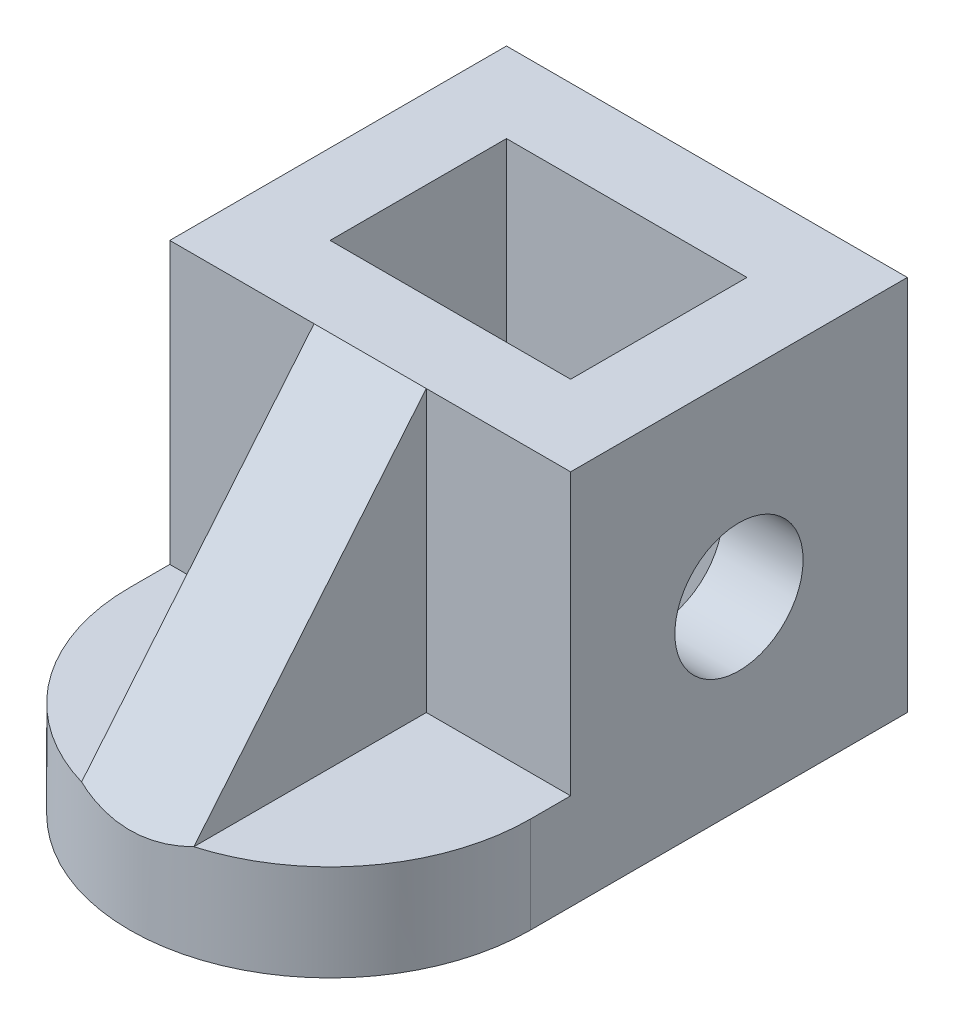
ISO-10303-21;
HEADER;
FILE_DESCRIPTION(('STEP AP214'),'2;1');
FILE_NAME('part.step','',(''),(''),'','','');
FILE_SCHEMA(('AUTOMOTIVE_DESIGN { 1 0 10303 214 1 1 1 1 }'));
ENDSEC;
DATA;
#1=APPLICATION_CONTEXT('core data for automotive mechanical design processes');
#2=APPLICATION_PROTOCOL_DEFINITION('international standard','automotive_design',2000,#1);
#3=PRODUCT_CONTEXT('',#1,'mechanical');
#4=PRODUCT('Part','Part','',(#3));
#5=PRODUCT_RELATED_PRODUCT_CATEGORY('part','',(#4));
#6=PRODUCT_DEFINITION_FORMATION('','',#4);
#7=PRODUCT_DEFINITION_CONTEXT('part definition',#1,'design');
#8=PRODUCT_DEFINITION('design','',#6,#7);
#9=PRODUCT_DEFINITION_SHAPE('','',#8);
#10=(LENGTH_UNIT() NAMED_UNIT(*) SI_UNIT(.MILLI.,.METRE.));
#11=(NAMED_UNIT(*) PLANE_ANGLE_UNIT() SI_UNIT($,.RADIAN.));
#12=(NAMED_UNIT(*) SI_UNIT($,.STERADIAN.) SOLID_ANGLE_UNIT());
#13=UNCERTAINTY_MEASURE_WITH_UNIT(LENGTH_MEASURE(1.E-05),#10,'distance_accuracy_value','');
#14=(GEOMETRIC_REPRESENTATION_CONTEXT(3) GLOBAL_UNCERTAINTY_ASSIGNED_CONTEXT((#13)) GLOBAL_UNIT_ASSIGNED_CONTEXT((#10,
#11,#12)) REPRESENTATION_CONTEXT('',''));
#15=CARTESIAN_POINT('',(0.,0.,0.));
#16=DIRECTION('',(0.,0.,1.));
#17=DIRECTION('',(1.,0.,0.));
#18=AXIS2_PLACEMENT_3D('',#15,#16,#17);
#19=CARTESIAN_POINT('',(-7.,23.5,15.));
#20=DIRECTION('',(1.,0.,0.));
#21=DIRECTION('',(0.,0.,-1.));
#22=AXIS2_PLACEMENT_3D('',#19,#20,#21);
#23=PLANE('',#22);
#24=DIRECTION('',(0.,-0.770021560905562,0.638017864750323));
#25=VECTOR('',#24,1.);
#26=CARTESIAN_POINT('',(-7.,12.,50.));
#27=LINE('',#26,#25);
#28=CARTESIAN_POINT('',(-7.,47.,21.));
#29=VERTEX_POINT('',#28);
#30=CARTESIAN_POINT('',(-7.,12.,50.));
#31=VERTEX_POINT('',#30);
#32=EDGE_CURVE('E146',#29,#31,#27,.T.);
#33=ORIENTED_EDGE('',*,*,#32,.F.);
#34=DIRECTION('',(0.,-1.,0.));
#35=VECTOR('',#34,1.);
#36=CARTESIAN_POINT('',(-7.,47.,21.));
#37=LINE('',#36,#35);
#38=CARTESIAN_POINT('',(-7.,12.,21.));
#39=VERTEX_POINT('',#38);
#40=EDGE_CURVE('E161',#29,#39,#37,.T.);
#41=ORIENTED_EDGE('',*,*,#40,.T.);
#42=DIRECTION('',(0.,0.,-1.));
#43=VECTOR('',#42,1.);
#44=CARTESIAN_POINT('',(-7.,12.,15.));
#45=LINE('',#44,#43);
#46=EDGE_CURVE('E56',#39,#31,#45,.F.);
#47=ORIENTED_EDGE('',*,*,#46,.T.);
#48=EDGE_LOOP('',(#33,#41,#47));
#49=FACE_BOUND('',#48,.T.);
#50=ADVANCED_FACE('F43',(#49),#23,.F.);
#51=CARTESIAN_POINT('',(7.,23.5,15.));
#52=DIRECTION('',(1.,0.,0.));
#53=DIRECTION('',(0.,0.,-1.));
#54=AXIS2_PLACEMENT_3D('',#51,#52,#53);
#55=PLANE('',#54);
#56=DIRECTION('',(0.,0.770021560905562,-0.638017864750323));
#57=VECTOR('',#56,1.);
#58=CARTESIAN_POINT('',(7.,12.,50.));
#59=LINE('',#58,#57);
#60=CARTESIAN_POINT('',(7.,12.,50.));
#61=VERTEX_POINT('',#60);
#62=CARTESIAN_POINT('',(7.,47.,21.));
#63=VERTEX_POINT('',#62);
#64=EDGE_CURVE('E158',#61,#63,#59,.T.);
#65=ORIENTED_EDGE('',*,*,#64,.F.);
#66=DIRECTION('',(0.,0.,-1.));
#67=VECTOR('',#66,1.);
#68=CARTESIAN_POINT('',(7.,12.,15.));
#69=LINE('',#68,#67);
#70=CARTESIAN_POINT('',(7.,12.,21.));
#71=VERTEX_POINT('',#70);
#72=EDGE_CURVE('E165',#71,#61,#69,.F.);
#73=ORIENTED_EDGE('',*,*,#72,.F.);
#74=DIRECTION('',(0.,-1.,0.));
#75=VECTOR('',#74,1.);
#76=CARTESIAN_POINT('',(7.,47.,21.));
#77=LINE('',#76,#75);
#78=EDGE_CURVE('E70',#63,#71,#77,.T.);
#79=ORIENTED_EDGE('',*,*,#78,.F.);
#80=EDGE_LOOP('',(#65,#73,#79));
#81=FACE_BOUND('',#80,.T.);
#82=ADVANCED_FACE('F279',(#81),#55,.T.);
#83=CARTESIAN_POINT('',(25.,47.,21.));
#84=DIRECTION('',(0.,0.,-1.));
#85=DIRECTION('',(-1.,0.,0.));
#86=AXIS2_PLACEMENT_3D('',#83,#84,#85);
#87=PLANE('',#86);
#88=ORIENTED_EDGE('',*,*,#40,.F.);
#89=DIRECTION('',(-1.,0.,0.));
#90=VECTOR('',#89,1.);
#91=CARTESIAN_POINT('',(25.,47.,21.));
#92=LINE('',#91,#90);
#93=CARTESIAN_POINT('',(-25.,47.,21.));
#94=VERTEX_POINT('',#93);
#95=EDGE_CURVE('E239',#29,#94,#92,.T.);
#96=ORIENTED_EDGE('',*,*,#95,.T.);
#97=DIRECTION('',(0.,-1.,0.));
#98=VECTOR('',#97,1.);
#99=CARTESIAN_POINT('',(-25.,47.,21.));
#100=LINE('',#99,#98);
#101=CARTESIAN_POINT('',(-25.,12.,21.));
#102=VERTEX_POINT('',#101);
#103=EDGE_CURVE('E234',#94,#102,#100,.T.);
#104=ORIENTED_EDGE('',*,*,#103,.T.);
#105=DIRECTION('',(-1.,0.,0.));
#106=VECTOR('',#105,1.);
#107=CARTESIAN_POINT('',(25.,12.,21.));
#108=LINE('',#107,#106);
#109=EDGE_CURVE('E228',#39,#102,#108,.T.);
#110=ORIENTED_EDGE('',*,*,#109,.F.);
#111=EDGE_LOOP('',(#88,#96,#104,#110));
#112=FACE_BOUND('',#111,.T.);
#113=ADVANCED_FACE('F288',(#112),#87,.F.);
#114=CARTESIAN_POINT('',(25.,12.,21.));
#115=DIRECTION('',(0.,-1.,0.));
#116=DIRECTION('',(0.,0.,-1.));
#117=AXIS2_PLACEMENT_3D('',#114,#115,#116);
#118=PLANE('',#117);
#119=ORIENTED_EDGE('',*,*,#46,.F.);
#120=ORIENTED_EDGE('',*,*,#109,.T.);
#121=DIRECTION('',(0.,0.,1.));
#122=VECTOR('',#121,1.);
#123=CARTESIAN_POINT('',(-25.,12.,21.));
#124=LINE('',#123,#122);
#125=CARTESIAN_POINT('',(-25.,12.,26.));
#126=VERTEX_POINT('',#125);
#127=EDGE_CURVE('E163',#102,#126,#124,.T.);
#128=ORIENTED_EDGE('',*,*,#127,.T.);
#129=CARTESIAN_POINT('',(0.,12.,26.));
#130=DIRECTION('',(0.,-1.,0.));
#131=DIRECTION('',(0.,0.,-1.));
#132=AXIS2_PLACEMENT_3D('',#129,#130,#131);
#133=CIRCLE('',#132,25.);
#134=EDGE_CURVE('E141',#126,#31,#133,.F.);
#135=ORIENTED_EDGE('',*,*,#134,.T.);
#136=EDGE_LOOP('',(#119,#120,#128,#135));
#137=FACE_BOUND('',#136,.T.);
#138=ADVANCED_FACE('F159',(#137),#118,.F.);
#139=CARTESIAN_POINT('',(25.,23.,0.));
#140=DIRECTION('',(-1.,0.,0.));
#141=DIRECTION('',(0.,0.,1.));
#142=AXIS2_PLACEMENT_3D('',#139,#140,#141);
#143=CYLINDRICAL_SURFACE('',#142,8.);
#144=CARTESIAN_POINT('',(15.,23.,0.));
#145=DIRECTION('',(1.,0.,0.));
#146=DIRECTION('',(0.,0.,-1.));
#147=AXIS2_PLACEMENT_3D('',#144,#145,#146);
#148=CIRCLE('',#147,8.);
#149=CARTESIAN_POINT('',(15.,23.,-8.));
#150=VERTEX_POINT('',#149);
#151=EDGE_CURVE('E179',#150,#150,#148,.F.);
#152=ORIENTED_EDGE('',*,*,#151,.T.);
#153=EDGE_LOOP('',(#152));
#154=FACE_BOUND('',#153,.T.);
#155=CARTESIAN_POINT('',(25.,23.,0.));
#156=DIRECTION('',(1.,0.,0.));
#157=DIRECTION('',(0.,0.,-1.));
#158=AXIS2_PLACEMENT_3D('',#155,#156,#157);
#159=CIRCLE('',#158,8.);
#160=CARTESIAN_POINT('',(25.,23.,-8.));
#161=VERTEX_POINT('',#160);
#162=EDGE_CURVE('E209',#161,#161,#159,.T.);
#163=ORIENTED_EDGE('',*,*,#162,.T.);
#164=EDGE_LOOP('',(#163));
#165=FACE_BOUND('',#164,.T.);
#166=ADVANCED_FACE('F321',(#154,#165),#143,.F.);
#167=CARTESIAN_POINT('',(0.,12.,26.));
#168=DIRECTION('',(0.,-1.,0.));
#169=DIRECTION('',(0.,0.,-1.));
#170=AXIS2_PLACEMENT_3D('',#167,#168,#169);
#171=CYLINDRICAL_SURFACE('',#170,25.);
#172=DIRECTION('',(0.,1.,0.));
#173=VECTOR('',#172,1.);
#174=CARTESIAN_POINT('',(25.,12.,26.));
#175=LINE('',#174,#173);
#176=CARTESIAN_POINT('',(25.,12.,26.));
#177=VERTEX_POINT('',#176);
#178=CARTESIAN_POINT('',(25.,0.,26.));
#179=VERTEX_POINT('',#178);
#180=EDGE_CURVE('E247',#177,#179,#175,.F.);
#181=ORIENTED_EDGE('',*,*,#180,.F.);
#182=EDGE_CURVE('E143',#61,#177,#133,.F.);
#183=ORIENTED_EDGE('',*,*,#182,.F.);
#184=CARTESIAN_POINT('',(0.,40.9655172413793,26.));
#185=DIRECTION('',(0.,-0.638017864750323,-0.770021560905562));
#186=DIRECTION('',(0.,-0.770021560905562,0.638017864750323));
#187=AXIS2_PLACEMENT_3D('',#184,#185,#186);
#188=ELLIPSE('',#187,39.1838557840121,25.);
#189=EDGE_CURVE('E11',#31,#61,#188,.F.);
#190=ORIENTED_EDGE('',*,*,#189,.F.);
#191=ORIENTED_EDGE('',*,*,#134,.F.);
#192=DIRECTION('',(0.,-1.,0.));
#193=VECTOR('',#192,1.);
#194=CARTESIAN_POINT('',(-25.,0.,26.));
#195=LINE('',#194,#193);
#196=CARTESIAN_POINT('',(-25.,0.,26.));
#197=VERTEX_POINT('',#196);
#198=EDGE_CURVE('E252',#197,#126,#195,.F.);
#199=ORIENTED_EDGE('',*,*,#198,.F.);
#200=CARTESIAN_POINT('',(0.,0.,26.));
#201=DIRECTION('',(0.,1.,0.));
#202=DIRECTION('',(0.,0.,1.));
#203=AXIS2_PLACEMENT_3D('',#200,#201,#202);
#204=CIRCLE('',#203,25.);
#205=EDGE_CURVE('E55',#179,#197,#204,.F.);
#206=ORIENTED_EDGE('',*,*,#205,.F.);
#207=EDGE_LOOP('',(#181,#183,#190,#191,#199,#206));
#208=FACE_BOUND('',#207,.T.);
#209=ADVANCED_FACE('F46',(#208),#171,.T.);
#210=CARTESIAN_POINT('',(25.,0.,0.));
#211=DIRECTION('',(1.,0.,0.));
#212=DIRECTION('',(0.,0.,-1.));
#213=AXIS2_PLACEMENT_3D('',#210,#211,#212);
#214=PLANE('',#213);
#215=DIRECTION('',(0.,0.,1.));
#216=VECTOR('',#215,1.);
#217=CARTESIAN_POINT('',(25.,12.,21.));
#218=LINE('',#217,#216);
#219=CARTESIAN_POINT('',(25.,12.,21.));
#220=VERTEX_POINT('',#219);
#221=EDGE_CURVE('E221',#220,#177,#218,.T.);
#222=ORIENTED_EDGE('',*,*,#221,.T.);
#223=ORIENTED_EDGE('',*,*,#180,.T.);
#224=DIRECTION('',(0.,0.,-1.));
#225=VECTOR('',#224,1.);
#226=CARTESIAN_POINT('',(25.,0.,51.));
#227=LINE('',#226,#225);
#228=CARTESIAN_POINT('',(25.,0.,-21.));
#229=VERTEX_POINT('',#228);
#230=EDGE_CURVE('E213',#179,#229,#227,.T.);
#231=ORIENTED_EDGE('',*,*,#230,.T.);
#232=DIRECTION('',(0.,1.,0.));
#233=VECTOR('',#232,1.);
#234=CARTESIAN_POINT('',(25.,0.,-21.));
#235=LINE('',#234,#233);
#236=CARTESIAN_POINT('',(25.,47.,-21.));
#237=VERTEX_POINT('',#236);
#238=EDGE_CURVE('E220',#229,#237,#235,.T.);
#239=ORIENTED_EDGE('',*,*,#238,.T.);
#240=DIRECTION('',(0.,0.,1.));
#241=VECTOR('',#240,1.);
#242=CARTESIAN_POINT('',(25.,47.,-21.));
#243=LINE('',#242,#241);
#244=CARTESIAN_POINT('',(25.,47.,21.));
#245=VERTEX_POINT('',#244);
#246=EDGE_CURVE('E217',#237,#245,#243,.T.);
#247=ORIENTED_EDGE('',*,*,#246,.T.);
#248=DIRECTION('',(0.,-1.,0.));
#249=VECTOR('',#248,1.);
#250=CARTESIAN_POINT('',(25.,47.,21.));
#251=LINE('',#250,#249);
#252=EDGE_CURVE('E223',#245,#220,#251,.T.);
#253=ORIENTED_EDGE('',*,*,#252,.T.);
#254=EDGE_LOOP('',(#222,#223,#231,#239,#247,#253));
#255=FACE_BOUND('',#254,.T.);
#256=ORIENTED_EDGE('',*,*,#162,.F.);
#257=EDGE_LOOP('',(#256));
#258=FACE_BOUND('',#257,.T.);
#259=ADVANCED_FACE('F269',(#255,#258),#214,.T.);
#260=CARTESIAN_POINT('',(-25.,0.,0.));
#261=DIRECTION('',(1.,0.,0.));
#262=DIRECTION('',(0.,0.,-1.));
#263=AXIS2_PLACEMENT_3D('',#260,#261,#262);
#264=PLANE('',#263);
#265=DIRECTION('',(0.,0.,-1.));
#266=VECTOR('',#265,1.);
#267=CARTESIAN_POINT('',(-25.,0.,51.));
#268=LINE('',#267,#266);
#269=CARTESIAN_POINT('',(-25.,0.,-21.));
#270=VERTEX_POINT('',#269);
#271=EDGE_CURVE('E215',#197,#270,#268,.T.);
#272=ORIENTED_EDGE('',*,*,#271,.F.);
#273=ORIENTED_EDGE('',*,*,#198,.T.);
#274=ORIENTED_EDGE('',*,*,#127,.F.);
#275=ORIENTED_EDGE('',*,*,#103,.F.);
#276=DIRECTION('',(0.,0.,1.));
#277=VECTOR('',#276,1.);
#278=CARTESIAN_POINT('',(-25.,47.,-21.));
#279=LINE('',#278,#277);
#280=CARTESIAN_POINT('',(-25.,47.,-21.));
#281=VERTEX_POINT('',#280);
#282=EDGE_CURVE('E233',#281,#94,#279,.T.);
#283=ORIENTED_EDGE('',*,*,#282,.F.);
#284=DIRECTION('',(0.,1.,0.));
#285=VECTOR('',#284,1.);
#286=CARTESIAN_POINT('',(-25.,0.,-21.));
#287=LINE('',#286,#285);
#288=EDGE_CURVE('E226',#270,#281,#287,.T.);
#289=ORIENTED_EDGE('',*,*,#288,.F.);
#290=EDGE_LOOP('',(#272,#273,#274,#275,#283,#289));
#291=FACE_BOUND('',#290,.T.);
#292=CARTESIAN_POINT('',(-25.,23.,0.));
#293=DIRECTION('',(1.,0.,0.));
#294=DIRECTION('',(0.,0.,-1.));
#295=AXIS2_PLACEMENT_3D('',#292,#293,#294);
#296=CIRCLE('',#295,8.);
#297=CARTESIAN_POINT('',(-25.,23.,-8.));
#298=VERTEX_POINT('',#297);
#299=EDGE_CURVE('E207',#298,#298,#296,.T.);
#300=ORIENTED_EDGE('',*,*,#299,.T.);
#301=EDGE_LOOP('',(#300));
#302=FACE_BOUND('',#301,.T.);
#303=ADVANCED_FACE('F256',(#291,#302),#264,.F.);
#304=CARTESIAN_POINT('',(25.,0.,51.));
#305=DIRECTION('',(0.,1.,0.));
#306=DIRECTION('',(0.,0.,1.));
#307=AXIS2_PLACEMENT_3D('',#304,#305,#306);
#308=PLANE('',#307);
#309=DIRECTION('',(-1.,0.,0.));
#310=VECTOR('',#309,1.);
#311=CARTESIAN_POINT('',(-15.,0.,11.));
#312=LINE('',#311,#310);
#313=CARTESIAN_POINT('',(15.,0.,11.));
#314=VERTEX_POINT('',#313);
#315=CARTESIAN_POINT('',(-15.,0.,11.));
#316=VERTEX_POINT('',#315);
#317=EDGE_CURVE('E173',#314,#316,#312,.T.);
#318=ORIENTED_EDGE('',*,*,#317,.F.);
#319=DIRECTION('',(0.,0.,1.));
#320=VECTOR('',#319,1.);
#321=CARTESIAN_POINT('',(15.,0.,-11.));
#322=LINE('',#321,#320);
#323=CARTESIAN_POINT('',(15.,0.,-11.));
#324=VERTEX_POINT('',#323);
#325=EDGE_CURVE('E176',#324,#314,#322,.T.);
#326=ORIENTED_EDGE('',*,*,#325,.F.);
#327=DIRECTION('',(1.,0.,0.));
#328=VECTOR('',#327,1.);
#329=CARTESIAN_POINT('',(-15.,0.,-11.));
#330=LINE('',#329,#328);
#331=CARTESIAN_POINT('',(-15.,0.,-11.));
#332=VERTEX_POINT('',#331);
#333=EDGE_CURVE('E196',#332,#324,#330,.T.);
#334=ORIENTED_EDGE('',*,*,#333,.F.);
#335=DIRECTION('',(0.,0.,-1.));
#336=VECTOR('',#335,1.);
#337=CARTESIAN_POINT('',(-15.,0.,-11.));
#338=LINE('',#337,#336);
#339=EDGE_CURVE('E171',#316,#332,#338,.T.);
#340=ORIENTED_EDGE('',*,*,#339,.F.);
#341=EDGE_LOOP('',(#318,#326,#334,#340));
#342=FACE_BOUND('',#341,.T.);
#343=ORIENTED_EDGE('',*,*,#230,.F.);
#344=ORIENTED_EDGE('',*,*,#205,.T.);
#345=ORIENTED_EDGE('',*,*,#271,.T.);
#346=DIRECTION('',(-1.,0.,0.));
#347=VECTOR('',#346,1.);
#348=CARTESIAN_POINT('',(25.,0.,-21.));
#349=LINE('',#348,#347);
#350=EDGE_CURVE('E244',#229,#270,#349,.T.);
#351=ORIENTED_EDGE('',*,*,#350,.F.);
#352=EDGE_LOOP('',(#343,#344,#345,#351));
#353=FACE_BOUND('',#352,.T.);
#354=ADVANCED_FACE('F251',(#342,#353),#308,.F.);
#355=CARTESIAN_POINT('',(25.,0.,-21.));
#356=DIRECTION('',(0.,0.,1.));
#357=DIRECTION('',(1.,0.,0.));
#358=AXIS2_PLACEMENT_3D('',#355,#356,#357);
#359=PLANE('',#358);
#360=ORIENTED_EDGE('',*,*,#288,.T.);
#361=DIRECTION('',(-1.,0.,0.));
#362=VECTOR('',#361,1.);
#363=CARTESIAN_POINT('',(25.,47.,-21.));
#364=LINE('',#363,#362);
#365=EDGE_CURVE('E243',#237,#281,#364,.T.);
#366=ORIENTED_EDGE('',*,*,#365,.F.);
#367=ORIENTED_EDGE('',*,*,#238,.F.);
#368=ORIENTED_EDGE('',*,*,#350,.T.);
#369=EDGE_LOOP('',(#360,#366,#367,#368));
#370=FACE_BOUND('',#369,.T.);
#371=ADVANCED_FACE('F264',(#370),#359,.F.);
#372=CARTESIAN_POINT('',(25.,47.,-21.));
#373=DIRECTION('',(0.,-1.,0.));
#374=DIRECTION('',(0.,0.,-1.));
#375=AXIS2_PLACEMENT_3D('',#372,#373,#374);
#376=PLANE('',#375);
#377=DIRECTION('',(0.,0.,1.));
#378=VECTOR('',#377,1.);
#379=CARTESIAN_POINT('',(-15.,47.,-11.));
#380=LINE('',#379,#378);
#381=CARTESIAN_POINT('',(-15.,47.,-11.));
#382=VERTEX_POINT('',#381);
#383=CARTESIAN_POINT('',(-15.,47.,11.));
#384=VERTEX_POINT('',#383);
#385=EDGE_CURVE('E190',#382,#384,#380,.T.);
#386=ORIENTED_EDGE('',*,*,#385,.F.);
#387=DIRECTION('',(-1.,0.,0.));
#388=VECTOR('',#387,1.);
#389=CARTESIAN_POINT('',(-15.,47.,-11.));
#390=LINE('',#389,#388);
#391=CARTESIAN_POINT('',(15.,47.,-11.));
#392=VERTEX_POINT('',#391);
#393=EDGE_CURVE('E184',#392,#382,#390,.T.);
#394=ORIENTED_EDGE('',*,*,#393,.F.);
#395=DIRECTION('',(0.,0.,-1.));
#396=VECTOR('',#395,1.);
#397=CARTESIAN_POINT('',(15.,47.,-11.));
#398=LINE('',#397,#396);
#399=CARTESIAN_POINT('',(15.,47.,11.));
#400=VERTEX_POINT('',#399);
#401=EDGE_CURVE('E182',#400,#392,#398,.T.);
#402=ORIENTED_EDGE('',*,*,#401,.F.);
#403=DIRECTION('',(1.,0.,0.));
#404=VECTOR('',#403,1.);
#405=CARTESIAN_POINT('',(-15.,47.,11.));
#406=LINE('',#405,#404);
#407=EDGE_CURVE('E188',#384,#400,#406,.T.);
#408=ORIENTED_EDGE('',*,*,#407,.F.);
#409=EDGE_LOOP('',(#386,#394,#402,#408));
#410=FACE_BOUND('',#409,.T.);
#411=ORIENTED_EDGE('',*,*,#365,.T.);
#412=ORIENTED_EDGE('',*,*,#282,.T.);
#413=ORIENTED_EDGE('',*,*,#95,.F.);
#414=EDGE_CURVE('E155',#63,#29,#92,.T.);
#415=ORIENTED_EDGE('',*,*,#414,.F.);
#416=EDGE_CURVE('E241',#245,#63,#92,.T.);
#417=ORIENTED_EDGE('',*,*,#416,.F.);
#418=ORIENTED_EDGE('',*,*,#246,.F.);
#419=EDGE_LOOP('',(#411,#412,#413,#415,#417,#418));
#420=FACE_BOUND('',#419,.T.);
#421=ADVANCED_FACE('F285',(#410,#420),#376,.F.);
#422=ORIENTED_EDGE('',*,*,#416,.T.);
#423=ORIENTED_EDGE('',*,*,#78,.T.);
#424=EDGE_CURVE('E238',#220,#71,#108,.T.);
#425=ORIENTED_EDGE('',*,*,#424,.F.);
#426=ORIENTED_EDGE('',*,*,#252,.F.);
#427=EDGE_LOOP('',(#422,#423,#425,#426));
#428=FACE_BOUND('',#427,.T.);
#429=ADVANCED_FACE('F283',(#428),#87,.F.);
#430=ORIENTED_EDGE('',*,*,#424,.T.);
#431=ORIENTED_EDGE('',*,*,#72,.T.);
#432=ORIENTED_EDGE('',*,*,#182,.T.);
#433=ORIENTED_EDGE('',*,*,#221,.F.);
#434=EDGE_LOOP('',(#430,#431,#432,#433));
#435=FACE_BOUND('',#434,.T.);
#436=ADVANCED_FACE('F273',(#435),#118,.F.);
#437=CARTESIAN_POINT('',(-15.,23.,0.));
#438=DIRECTION('',(-1.,0.,0.));
#439=DIRECTION('',(0.,0.,1.));
#440=AXIS2_PLACEMENT_3D('',#437,#438,#439);
#441=CIRCLE('',#440,8.);
#442=CARTESIAN_POINT('',(-15.,23.,8.));
#443=VERTEX_POINT('',#442);
#444=EDGE_CURVE('E177',#443,#443,#441,.F.);
#445=ORIENTED_EDGE('',*,*,#444,.T.);
#446=EDGE_LOOP('',(#445));
#447=FACE_BOUND('',#446,.T.);
#448=ORIENTED_EDGE('',*,*,#299,.F.);
#449=EDGE_LOOP('',(#448));
#450=FACE_BOUND('',#449,.T.);
#451=ADVANCED_FACE('F293',(#447,#450),#143,.F.);
#452=CARTESIAN_POINT('',(15.,-0.001000000000001,-11.));
#453=DIRECTION('',(1.,0.,0.));
#454=DIRECTION('',(0.,0.,-1.));
#455=AXIS2_PLACEMENT_3D('',#452,#453,#454);
#456=PLANE('',#455);
#457=ORIENTED_EDGE('',*,*,#151,.F.);
#458=EDGE_LOOP('',(#457));
#459=FACE_BOUND('',#458,.T.);
#460=ORIENTED_EDGE('',*,*,#325,.T.);
#461=DIRECTION('',(0.,1.,0.));
#462=VECTOR('',#461,1.);
#463=CARTESIAN_POINT('',(15.,-0.00100000000001488,11.));
#464=LINE('',#463,#462);
#465=EDGE_CURVE('E194',#314,#400,#464,.T.);
#466=ORIENTED_EDGE('',*,*,#465,.T.);
#467=ORIENTED_EDGE('',*,*,#401,.T.);
#468=DIRECTION('',(0.,1.,0.));
#469=VECTOR('',#468,1.);
#470=CARTESIAN_POINT('',(15.,-0.001000000000001,-11.));
#471=LINE('',#470,#469);
#472=EDGE_CURVE('E195',#324,#392,#471,.T.);
#473=ORIENTED_EDGE('',*,*,#472,.F.);
#474=EDGE_LOOP('',(#460,#466,#467,#473));
#475=FACE_BOUND('',#474,.T.);
#476=ADVANCED_FACE('F309',(#459,#475),#456,.F.);
#477=CARTESIAN_POINT('',(-15.,-0.00100000000001488,11.));
#478=DIRECTION('',(0.,0.,1.));
#479=DIRECTION('',(0.,-1.,0.));
#480=AXIS2_PLACEMENT_3D('',#477,#478,#479);
#481=PLANE('',#480);
#482=ORIENTED_EDGE('',*,*,#407,.T.);
#483=ORIENTED_EDGE('',*,*,#465,.F.);
#484=ORIENTED_EDGE('',*,*,#317,.T.);
#485=DIRECTION('',(0.,1.,0.));
#486=VECTOR('',#485,1.);
#487=CARTESIAN_POINT('',(-15.,-0.00100000000001488,11.));
#488=LINE('',#487,#486);
#489=EDGE_CURVE('E200',#316,#384,#488,.T.);
#490=ORIENTED_EDGE('',*,*,#489,.T.);
#491=EDGE_LOOP('',(#482,#483,#484,#490));
#492=FACE_BOUND('',#491,.T.);
#493=ADVANCED_FACE('F306',(#492),#481,.F.);
#494=CARTESIAN_POINT('',(-15.,-0.001000000000001,-11.));
#495=DIRECTION('',(-1.,0.,0.));
#496=DIRECTION('',(0.,0.,1.));
#497=AXIS2_PLACEMENT_3D('',#494,#495,#496);
#498=PLANE('',#497);
#499=ORIENTED_EDGE('',*,*,#444,.F.);
#500=EDGE_LOOP('',(#499));
#501=FACE_BOUND('',#500,.T.);
#502=ORIENTED_EDGE('',*,*,#339,.T.);
#503=DIRECTION('',(0.,1.,0.));
#504=VECTOR('',#503,1.);
#505=CARTESIAN_POINT('',(-15.,-0.001000000000001,-11.));
#506=LINE('',#505,#504);
#507=EDGE_CURVE('E197',#332,#382,#506,.T.);
#508=ORIENTED_EDGE('',*,*,#507,.T.);
#509=ORIENTED_EDGE('',*,*,#385,.T.);
#510=ORIENTED_EDGE('',*,*,#489,.F.);
#511=EDGE_LOOP('',(#502,#508,#509,#510));
#512=FACE_BOUND('',#511,.T.);
#513=ADVANCED_FACE('F307',(#501,#512),#498,.F.);
#514=CARTESIAN_POINT('',(-15.,-0.001000000000001,-11.));
#515=DIRECTION('',(0.,0.,-1.));
#516=DIRECTION('',(0.,1.,0.));
#517=AXIS2_PLACEMENT_3D('',#514,#515,#516);
#518=PLANE('',#517);
#519=ORIENTED_EDGE('',*,*,#393,.T.);
#520=ORIENTED_EDGE('',*,*,#507,.F.);
#521=ORIENTED_EDGE('',*,*,#333,.T.);
#522=ORIENTED_EDGE('',*,*,#472,.T.);
#523=EDGE_LOOP('',(#519,#520,#521,#522));
#524=FACE_BOUND('',#523,.T.);
#525=ADVANCED_FACE('F313',(#524),#518,.F.);
#526=CARTESIAN_POINT('',(-25.001,12.,50.));
#527=DIRECTION('',(0.,-0.638017864750323,-0.770021560905562));
#528=DIRECTION('',(0.,0.770021560905562,-0.638017864750323));
#529=AXIS2_PLACEMENT_3D('',#526,#527,#528);
#530=PLANE('',#529);
#531=ORIENTED_EDGE('',*,*,#32,.T.);
#532=ORIENTED_EDGE('',*,*,#189,.T.);
#533=ORIENTED_EDGE('',*,*,#64,.T.);
#534=ORIENTED_EDGE('',*,*,#414,.T.);
#535=EDGE_LOOP('',(#531,#532,#533,#534));
#536=FACE_BOUND('',#535,.T.);
#537=ADVANCED_FACE('F148',(#536),#530,.F.);
#538=CLOSED_SHELL('',(#50,#82,#113,#138,#166,#209,#259,#303,#354,#371,#421,#429,#436,#451,#476,
#493,#513,#525,#537));
#539=MANIFOLD_SOLID_BREP('B2',#538);
#540=ADVANCED_BREP_SHAPE_REPRESENTATION('',(#18,#539),#14);
#541=SHAPE_DEFINITION_REPRESENTATION(#9,#540);
ENDSEC;
END-ISO-10303-21;
